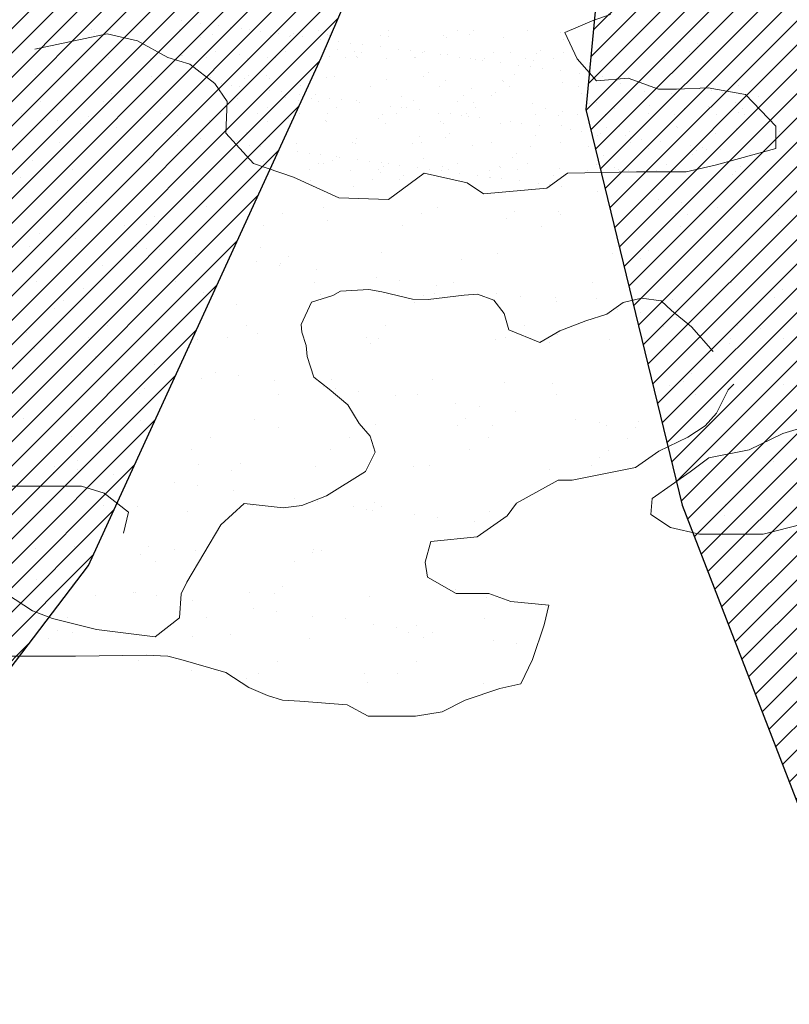
# Model space of a CAD drawing. Units: inches. Extents: x 1986 to 21484, y -1816 to 2016.
# Tile 13 of 85: x 2165 to 2172, y 1865 to 1874. Entities that reach past the tile are written whole.
import ezdxf

# ---------------------------------------------------------------- set-up
doc = ezdxf.new("R2010")
doc.units = ezdxf.units.IN
doc.layers.add('L-PLNT', color=84, linetype='Continuous', lineweight=13)
doc.layers.add('vfolhas', color=114, linetype='Continuous', lineweight=5)
for name, color, linetype in [('vfolha', 72, 'Continuous'), ('vfolha2', 110, 'Continuous'), ('vfolhas2', 102, 'Continuous')]:
    doc.layers.add(name, color=color, linetype=linetype)
pattern_1 = [(45, (-2446.5133113, 50.986076), (-0.004419417382, 0.004419417382), [])]

# ---------------------------------------------------------------- blocks, each defined once
blk = doc.blocks.new('arbusto_PB_verde_grande')
at = {"layer": 'vfolha2'}
h = blk.add_hatch(dxfattribs=at)
h.set_pattern_fill('ANSI31', color=256, scale=0.05, style=0)
h.set_pattern_definition(pattern_1)
h.paths.add_polyline_path([(0.02944, 0.35651), (0.00028, 0.09048), (0.02625, -0.03934), (0.047, 0.06233), (0.06189, 0.09731), (0.09372, 0.26573), (0.09955, 0.43473), (0.08789, 0.61313), (0.0645, 0.72266), (0.04988, 0.6851), (0.0236, 0.51294)])
h.paths.add_polyline_path([(0.30106, 0.43789), (0.14225, 0.24871), (0.26685, 0.30022)])
h.paths.add_polyline_path([(0.37995, 0.22817), (0.23697, 0.15193), (0.18428, 0.09364), (0.11122, 0.04358), (0.02625, -0.03934), (0.28061, 0.04667), (0.36829, 0.07798), (0.46756, 0.11239), (0.61068, 0.19376), (0.71585, 0.27823), (0.55813, 0.25948)])
h.paths.add_polyline_path([(0.56101, -0.29441), (0.72752, -0.32573), (0.59024, -0.2412), (0.42962, -0.15982), (0.02625, -0.03934), (0.14922, -0.14107), (0.18838, -0.16604), (0.41501, -0.24435)])
h.paths.add_polyline_path([(-0.27429, -0.44776), (-0.30352, -0.72628), (-0.23923, -0.64175), (-0.15457, -0.45716), (0.02625, -0.03934), (-0.16328, -0.25376)])
h.paths.add_polyline_path([(-0.51963, -0.24744), (-0.67736, -0.32573), (-0.59558, -0.35072), (-0.40574, -0.32882), (-0.21007, -0.20995), (0.02625, -0.03934), (-0.14874, -0.06595), (-0.31518, -0.09101), (-0.41452, -0.15048)])
h.paths.add_polyline_path([(-0.52546, 0.25007), (-0.70947, 0.24698), (-0.51963, 0.1093), (-0.32979, 0.02167), (-0.07567, -0.0128), (-0.04234, -0.02148), (-0.35024, 0.1312)])
at = {"layer": 'vfolhas'}
h = blk.add_hatch(dxfattribs=at)
h.set_pattern_fill('ANSI31', color=256, scale=0.05, style=0)
h.set_pattern_definition(pattern_1)
h.paths.add_polyline_path([(-0.07279, 0.50669), (-0.18085, 0.65063), (-0.2334, 0.67253), (-0.20712, 0.53176), (-0.10785, 0.25007), (0.02625, -0.03934), (0.00028, 0.09048), (0.00816, 0.16241), (-0.04939, 0.29079)])
h.paths.add_polyline_path([(0.09902, 0.41929), (0.09372, 0.26573), (0.07906, 0.18814), (0.15506, 0.36901), (0.26606, 0.5505), (0.28356, 0.63504), (0.2485, 0.68819), (0.25145, 0.63504), (0.20178, 0.54426)])
h.paths.add_polyline_path([(0.12295, 0.24073), (0.047, 0.06233), (0.02625, -0.03934), (0.11122, 0.04358), (0.18428, 0.09364), (0.27478, 0.19376), (0.3215, 0.25323), (0.44129, 0.38467), (0.47634, 0.57866), (0.41789, 0.45347), (0.28939, 0.30954)])
h.paths.add_polyline_path([(0.58145, -0.03779), (0.70707, 0.01536), (0.78591, 0.04667), (0.74796, 0.06549), (0.62818, 0.08423), (0.52595, 0.09048), (0.39745, 0.04358), (0.02625, -0.03934), (0.25728, -0.03154), (0.43834, -0.0347)])
h.paths.add_polyline_path([(0.52022, -0.03647), (0.43834, -0.0347), (0.25728, -0.03154), (0.02625, -0.03934), (0.17964, -0.08515), (0.53768, -0.13167), (0.69541, -0.15357), (0.78591, -0.07852), (0.70413, -0.10042)])
h.paths.add_polyline_path([(0.27189, -0.21929), (0.14922, -0.14107), (0.02625, -0.03934), (0.15794, -0.31007), (0.29522, -0.42585), (0.41789, -0.49157), (0.56396, -0.56669), (0.5114, -0.48532), (0.39456, -0.34139)])
h.paths.add_polyline_path([(-0.05818, -0.47591), (-0.02312, -0.61984), (0.047, -0.80134), (0.08494, -0.59794), (0.07911, -0.4071), (0.03527, -0.25376), (0.02625, -0.03934), (-0.03773, -0.26001)])
h.paths.add_polyline_path([(-0.24218, 0.14054), (-0.11073, 0.06858), (0.02625, -0.03934), (-0.04235, 0.10871), (-0.21007, 0.23757), (-0.36485, 0.33145), (-0.47874, 0.40341), (-0.54303, 0.46288), (-0.49041, 0.33145), (-0.39408, 0.22192)])
at = {"layer": 'vfolha'}
for p, q in [((-0.03773, -0.26001), (-0.05818, -0.47591)), ((-0.02312, -0.61984), (0.047, -0.80134))]:
    blk.add_line(p, q, dxfattribs=at)
at = {"layer": 'vfolha2'}
for p, q in [((-0.15457, -0.45716), (0.02625, -0.03934)), ((-0.30352, -0.72628), (-0.23923, -0.64175))]:
    blk.add_line(p, q, dxfattribs=at)
at = {"layer": 'vfolhas2'}
for p, q in [((-0.23923, -0.64175), (-0.15457, -0.45716)), ((-0.05818, -0.47591), (-0.02312, -0.61984))]:
    blk.add_line(p, q, dxfattribs=at)
blk = doc.blocks.new('PLANT-SHRUB')
for p, q in [((2166.5746, 1873.8887), (2166.5746, 1873.8887)), ((2170.0035, 1873.7837), (2170.2627, 1873.8946)), ((2170.2627, 1873.8946), (2170.4108, 1873.944)), ((2165.7672, 1873.807), (2165.7672, 1873.807)), ((2165.9347, 1873.8098), (2165.9347, 1873.8098)), ((2166.557, 1873.8087), (2166.557, 1873.8087)), ((2166.737, 1873.8673), (2166.737, 1873.8673)), ((2166.9045, 1873.8453), (2166.9045, 1873.8453)), ((2167.0085, 1873.8316), (2167.0085, 1873.8316)), ((2167.1125, 1873.8179), (2167.1125, 1873.8179)), ((2167.1125, 1873.8179), (2167.1125, 1873.8179)), ((2167.1794, 1873.8075), (2167.1794, 1873.8075)), ((2167.2749, 1873.7965), (2167.2749, 1873.7965)), ((2167.8017, 1873.8064), (2167.8017, 1873.8064)), ((2168.424, 1873.8053), (2168.424, 1873.8053)), ((2169.0463, 1873.8041), (2169.0463, 1873.8041)), ((2169.1885, 1873.8023), (2169.1885, 1873.8023)), ((2169.6686, 1873.803), (2169.6686, 1873.803)), ((2165.2583, 1873.6357), (2165.9062, 1873.7713)), ((2165.7957, 1873.7851), (2165.7957, 1873.7851)), ((2165.9062, 1873.7713), (2166.1777, 1873.7097)), ((2166.1777, 1873.7097), (2166.4493, 1873.5617)), ((2166.1777, 1873.7097), (2166.1777, 1873.7097)), ((2166.3069, 1873.7875), (2166.3069, 1873.7875)), ((2166.741, 1873.7371), (2166.741, 1873.7371)), ((2166.8467, 1873.7681), (2166.8467, 1873.7681)), ((2166.8467, 1873.7681), (2166.8467, 1873.7681)), ((2167.3697, 1873.7614), (2167.3697, 1873.7614)), ((2167.4374, 1873.7751), (2167.4374, 1873.7751)), ((2167.5406, 1873.744), (2167.5406, 1873.744)), ((2167.5464, 1873.7608), (2167.5464, 1873.7608)), ((2167.5774, 1873.7777), (2167.5774, 1873.7777)), ((2167.6504, 1873.7471), (2167.6504, 1873.7471)), ((2167.8129, 1873.7257), (2167.8129, 1873.7257)), ((2167.8809, 1873.7638), (2167.8809, 1873.7638)), ((2167.8928, 1873.7547), (2167.8928, 1873.7547)), ((2168.352, 1873.7617), (2168.352, 1873.7617)), ((2168.4207, 1873.7444), (2168.4207, 1873.7444)), ((2168.9152, 1873.7596), (2168.9152, 1873.7596)), ((2168.9438, 1873.7377), (2168.9438, 1873.7377)), ((2169.1516, 1873.7685), (2169.1516, 1873.7685)), ((2169.455, 1873.7402), (2169.455, 1873.7402)), ((2169.9631, 1873.7862), (2169.9631, 1873.7862)), ((2169.9947, 1873.7207), (2169.9947, 1873.7207)), ((2169.9947, 1873.7207), (2169.9947, 1873.7207)), ((2170.1146, 1873.5494), (2170.0035, 1873.7837)), ((2167.9692, 1873.6361), (2167.9692, 1873.6361)), ((2167.9803, 1873.7037), (2167.9803, 1873.7037)), ((2168.0843, 1873.69), (2168.0843, 1873.69)), ((2168.1883, 1873.6763), (2168.1883, 1873.6763)), ((2168.1883, 1873.6763), (2168.1883, 1873.6763)), ((2168.3508, 1873.6549), (2168.3508, 1873.6549)), ((2168.5132, 1873.6335), (2168.5132, 1873.6335)), ((2169.7892, 1873.6269), (2169.7892, 1873.6269)), ((2171.0409, 1873.7074), (2171.0409, 1873.7074)), ((2171.1913, 1873.6852), (2171.1913, 1873.6852)), ((2165.9152, 1873.5563), (2165.9152, 1873.5563)), ((2166.2963, 1873.5549), (2166.2963, 1873.5549)), ((2166.4493, 1873.5617), (2166.6467, 1873.5)), ((2166.5303, 1873.5441), (2166.5303, 1873.5441)), ((2166.5671, 1873.5778), (2166.5671, 1873.5778)), ((2166.5764, 1873.5807), (2166.5764, 1873.5807)), ((2166.7917, 1873.5606), (2166.7917, 1873.5606)), ((2166.876, 1873.6143), (2166.876, 1873.6143)), ((2167.0876, 1873.5831), (2167.0876, 1873.5831)), ((2167.1598, 1873.5541), (2167.1598, 1873.5541)), ((2167.3417, 1873.5617), (2167.3417, 1873.5617)), ((2167.414, 1873.5594), (2167.414, 1873.5594)), ((2167.4983, 1873.6131), (2167.4983, 1873.6131)), ((2167.6274, 1873.5637), (2167.6274, 1873.5637)), ((2167.8955, 1873.5686), (2167.8955, 1873.5686)), ((2168.0363, 1873.5583), (2168.0363, 1873.5583)), ((2168.1206, 1873.612), (2168.1206, 1873.612)), ((2168.1413, 1873.5686), (2168.1413, 1873.5686)), ((2168.1505, 1873.557), (2168.1505, 1873.557)), ((2168.1782, 1873.6023), (2168.1782, 1873.6023)), ((2168.4044, 1873.5518), (2168.4044, 1873.5518)), ((2168.6222, 1873.6192), (2168.6222, 1873.6192)), ((2168.6587, 1873.5572), (2168.6587, 1873.5572)), ((2168.6617, 1873.5595), (2168.6617, 1873.5595)), ((2168.7262, 1873.6055), (2168.7262, 1873.6055)), ((2168.7429, 1873.6109), (2168.7429, 1873.6109)), ((2168.8887, 1873.5841), (2168.8887, 1873.5841)), ((2168.9527, 1873.5863), (2168.9527, 1873.5863)), ((2169.0561, 1873.562), (2169.0561, 1873.562)), ((2169.1601, 1873.5483), (2169.1601, 1873.5483)), ((2169.2014, 1873.54), (2169.2014, 1873.54)), ((2169.2641, 1873.5346), (2169.2641, 1873.5346)), ((2169.2641, 1873.5346), (2169.2641, 1873.5346)), ((2169.281, 1873.556), (2169.281, 1873.556)), ((2169.3653, 1873.6097), (2169.3653, 1873.6097)), ((2169.5184, 1873.6039), (2169.5184, 1873.6039)), ((2169.6491, 1873.5495), (2169.6491, 1873.5495)), ((2169.7245, 1873.5334), (2169.7245, 1873.5334)), ((2169.7524, 1873.5931), (2169.7524, 1873.5931)), ((2169.9033, 1873.5549), (2169.9033, 1873.5549)), ((2169.9876, 1873.6086), (2169.9876, 1873.6086)), ((2170.1146, 1873.5494), (2170.1146, 1873.5494)), ((2170.2874, 1873.352), (2170.1146, 1873.5494)), ((2170.8937, 1873.5473), (2170.8937, 1873.5473)), ((2171.1176, 1873.6177), (2171.1176, 1873.6177)), ((2166.6467, 1873.5), (2166.8689, 1873.3274)), ((2169.4266, 1873.5133), (2169.4266, 1873.5133)), ((2169.5891, 1873.4919), (2169.5891, 1873.4919)), ((2169.698, 1873.4775), (2169.698, 1873.4775)), ((2169.802, 1873.4638), (2169.802, 1873.4638)), ((2165.2601, 1873.4067), (2165.2601, 1873.4067)), ((2166.3062, 1873.3933), (2166.3062, 1873.3933)), ((2166.8341, 1873.383), (2166.8341, 1873.383)), ((2167.131, 1873.3687), (2167.131, 1873.3687)), ((2167.1678, 1873.4024), (2167.1678, 1873.4024)), ((2167.3286, 1873.3982), (2167.3286, 1873.3982)), ((2167.3572, 1873.3763), (2167.3572, 1873.3763)), ((2167.8684, 1873.3788), (2167.8684, 1873.3788)), ((2167.9424, 1873.3863), (2167.9424, 1873.3863)), ((2168.4081, 1873.3593), (2168.4081, 1873.3593)), ((2168.4081, 1873.3593), (2168.4081, 1873.3593)), ((2168.742, 1873.3932), (2168.742, 1873.3932)), ((2168.7789, 1873.427), (2168.7789, 1873.427)), ((2169.5535, 1873.4109), (2169.5535, 1873.4109)), ((2169.9645, 1873.4424), (2169.9645, 1873.4424)), ((2170.1319, 1873.4204), (2170.1319, 1873.4204)), ((2170.2359, 1873.4067), (2170.2359, 1873.4067)), ((2170.5712, 1873.3767), (2170.2874, 1873.352)), ((2170.34, 1873.393), (2170.34, 1873.393)), ((2170.8427, 1873.2781), (2170.5712, 1873.3767)), ((2166.8689, 1873.3274), (2166.9799, 1873.1671)), ((2166.9282, 1873.3248), (2166.9282, 1873.3248)), ((2167.018, 1873.3071), (2167.018, 1873.3071)), ((2167.0907, 1873.3034), (2167.0907, 1873.3034)), ((2167.3621, 1873.2676), (2167.3621, 1873.2676)), ((2167.6403, 1873.306), (2167.6403, 1873.306)), ((2168.2626, 1873.3049), (2168.2626, 1873.3049)), ((2168.8849, 1873.3037), (2168.8849, 1873.3037)), ((2168.9312, 1873.3527), (2168.9312, 1873.3527)), ((2169.1706, 1873.2853), (2169.1706, 1873.2853)), ((2169.4424, 1873.3551), (2169.4424, 1873.3551)), ((2169.4543, 1873.346), (2169.4543, 1873.346)), ((2169.5072, 1873.3026), (2169.5072, 1873.3026)), ((2169.9821, 1873.3357), (2169.9821, 1873.3357)), ((2170.1295, 1873.3015), (2170.1295, 1873.3015)), ((2170.4767, 1873.3509), (2170.4767, 1873.3509)), ((2170.5052, 1873.329), (2170.5052, 1873.329)), ((2170.6649, 1873.3502), (2170.6649, 1873.3502)), ((2170.7519, 1873.3003), (2170.7519, 1873.3003)), ((2171.0032, 1873.2781), (2170.8427, 1873.2781)), ((2170.9907, 1873.2761), (2170.9907, 1873.2761)), ((2171.287, 1873.2904), (2171.0032, 1873.2781)), ((2171.2077, 1873.2788), (2171.2077, 1873.2788)), ((2171.6202, 1873.2287), (2171.287, 1873.2904)), ((2171.5561, 1873.312), (2171.5561, 1873.312)), ((2165.9485, 1873.2362), (2165.9485, 1873.2362)), ((2167.0751, 1873.1981), (2167.0751, 1873.1981)), ((2167.4661, 1873.254), (2167.4661, 1873.254)), ((2167.4977, 1873.2041), (2167.4977, 1873.2041)), ((2167.6286, 1873.2326), (2167.6286, 1873.2326)), ((2167.7317, 1873.1933), (2167.7317, 1873.1933)), ((2167.7686, 1873.227), (2167.7686, 1873.227)), ((2167.9, 1873.1968), (2167.9, 1873.1968)), ((2168.0041, 1873.1831), (2168.0041, 1873.1831)), ((2168.5431, 1873.2109), (2168.5431, 1873.2109)), ((2169.097, 1873.2178), (2169.097, 1873.2178)), ((2169.3428, 1873.2178), (2169.3428, 1873.2178)), ((2169.3796, 1873.2516), (2169.3796, 1873.2516)), ((2170.1542, 1873.2355), (2170.1542, 1873.2355)), ((2170.7198, 1873.2532), (2170.7198, 1873.2532)), ((2170.9538, 1873.2424), (2170.9538, 1873.2424)), ((2171.3118, 1873.2651), (2171.3118, 1873.2651)), ((2171.4158, 1873.2514), (2171.4158, 1873.2514)), ((2171.4158, 1873.2514), (2171.4158, 1873.2514)), ((2171.5782, 1873.23), (2171.5782, 1873.23)), ((2171.8918, 1872.9451), (2171.6202, 1873.2287)), ((2171.7407, 1873.2086), (2171.7407, 1873.2086)), ((2165.3084, 1873.1698), (2165.3084, 1873.1698)), ((2165.8749, 1873.1687), (2165.8749, 1873.1687)), ((2166.5531, 1873.1675), (2166.5531, 1873.1675)), ((2166.9799, 1873.1671), (2166.9676, 1872.8834)), ((2167.3369, 1873.1127), (2167.3369, 1873.1127)), ((2167.6148, 1873.1787), (2167.6148, 1873.1787)), ((2167.7977, 1873.1653), (2167.7977, 1873.1653)), ((2167.9592, 1873.1116), (2167.9592, 1873.1116)), ((2168.1379, 1873.172), (2168.1379, 1873.172)), ((2168.1665, 1873.1617), (2168.1665, 1873.1617)), ((2168.438, 1873.126), (2168.438, 1873.126)), ((2168.542, 1873.1123), (2168.542, 1873.1123)), ((2168.5815, 1873.1105), (2168.5815, 1873.1105)), ((2168.6491, 1873.1744), (2168.6491, 1873.1744)), ((2168.7044, 1873.0909), (2168.7044, 1873.0909)), ((2169.0423, 1873.163), (2169.0423, 1873.163)), ((2169.1888, 1873.155), (2169.1888, 1873.155)), ((2169.2039, 1873.1093), (2169.2039, 1873.1093)), ((2169.7119, 1873.1483), (2169.7119, 1873.1483)), ((2169.8262, 1873.1082), (2169.8262, 1873.1082)), ((2170.2231, 1873.1508), (2170.2231, 1873.1508)), ((2170.287, 1873.1607), (2170.287, 1873.1607)), ((2170.4485, 1873.1071), (2170.4485, 1873.1071)), ((2170.7628, 1873.1313), (2170.7628, 1873.1313)), ((2171.0708, 1873.1059), (2171.0708, 1873.1059)), ((2171.2859, 1873.1247), (2171.2859, 1873.1247)), ((2171.5316, 1873.1585), (2171.5316, 1873.1585)), ((2171.5914, 1873.1007), (2171.5914, 1873.1007)), ((2165.1399, 1873.0624), (2165.1399, 1873.0624)), ((2165.742, 1873.0369), (2165.742, 1873.0369)), ((2166.3845, 1873.0602), (2166.3845, 1873.0602)), ((2167.2526, 1873.059), (2167.2526, 1873.059)), ((2167.5328, 1873.011), (2167.5328, 1873.011)), ((2167.6292, 1873.0579), (2167.6292, 1873.0579)), ((2167.875, 1873.0579), (2167.875, 1873.0579)), ((2168.3325, 1873.0179), (2168.3325, 1873.0179)), ((2168.3693, 1873.0516), (2168.3693, 1873.0516)), ((2168.4973, 1873.0568), (2168.4973, 1873.0568)), ((2168.8738, 1873.0556), (2168.8738, 1873.0556)), ((2168.9759, 1873.0552), (2168.9759, 1873.0552)), ((2169.0799, 1873.0415), (2169.0799, 1873.0415)), ((2169.1196, 1873.0556), (2169.1196, 1873.0556)), ((2169.1439, 1873.0356), (2169.1439, 1873.0356)), ((2169.2423, 1873.0201), (2169.2423, 1873.0201)), ((2169.7419, 1873.0545), (2169.7419, 1873.0545)), ((2169.9435, 1873.0424), (2169.9435, 1873.0424)), ((2169.9803, 1873.0762), (2169.9803, 1873.0762)), ((2170.1184, 1873.0534), (2170.1184, 1873.0534)), ((2170.3642, 1873.0534), (2170.3642, 1873.0534)), ((2170.7549, 1873.0601), (2170.7549, 1873.0601)), ((2170.9865, 1873.0522), (2170.9865, 1873.0522)), ((2171.3631, 1873.0511), (2171.3631, 1873.0511)), ((2171.5546, 1873.067), (2171.5546, 1873.067)), ((2171.6089, 1873.0511), (2171.6089, 1873.0511)), ((2165.4601, 1873.0006), (2165.4601, 1873.0006)), ((2165.6682, 1872.9733), (2165.6682, 1872.9733)), ((2165.9931, 1872.9305), (2165.9931, 1872.9305)), ((2166.8215, 1872.998), (2166.8215, 1872.998)), ((2167.3446, 1872.9913), (2167.3446, 1872.9913)), ((2167.8558, 1872.9937), (2167.8558, 1872.9937)), ((2167.8677, 1872.9846), (2167.8677, 1872.9846)), ((2168.3955, 1872.9743), (2168.3955, 1872.9743)), ((2168.8901, 1872.9895), (2168.8901, 1872.9895)), ((2168.9186, 1872.9676), (2168.9186, 1872.9676)), ((2169.4298, 1872.9701), (2169.4298, 1872.9701)), ((2169.5138, 1872.9844), (2169.5138, 1872.9844)), ((2169.6178, 1872.9707), (2169.6178, 1872.9707)), ((2169.7803, 1872.9493), (2169.7803, 1872.9493)), ((2169.9695, 1872.9506), (2169.9695, 1872.9506)), ((2169.9695, 1872.9506), (2169.9695, 1872.9506)), ((2170.3721, 1872.9345), (2170.3721, 1872.9345)), ((2170.4926, 1872.944), (2170.4926, 1872.944)), ((2171.0038, 1872.9464), (2171.0038, 1872.9464)), ((2171.0157, 1872.9373), (2171.0157, 1872.9373)), ((2171.5435, 1872.927), (2171.5435, 1872.927)), ((2171.8918, 1872.7478), (2171.8918, 1872.9451)), ((2166.536, 1872.859), (2166.536, 1872.859)), ((2166.744, 1872.8316), (2166.744, 1872.8316)), ((2166.9676, 1872.8834), (2167.2144, 1872.6121)), ((2167.15, 1872.8855), (2167.15, 1872.8855)), ((2167.359, 1872.8517), (2167.359, 1872.8517)), ((2168.1336, 1872.8356), (2168.1336, 1872.8356)), ((2168.6992, 1872.8533), (2168.6992, 1872.8533)), ((2168.9332, 1872.8425), (2168.9332, 1872.8425)), ((2168.97, 1872.8762), (2168.97, 1872.8762)), ((2169.7446, 1872.8602), (2169.7446, 1872.8602)), ((2170.0517, 1872.9136), (2170.0517, 1872.9136)), ((2170.1557, 1872.8999), (2170.1557, 1872.8999)), ((2170.2984, 1872.867), (2170.2984, 1872.867)), ((2170.3182, 1872.8785), (2170.3182, 1872.8785)), ((2170.5442, 1872.867), (2170.5442, 1872.867)), ((2170.5811, 1872.9008), (2170.5811, 1872.9008)), ((2170.5896, 1872.8427), (2170.5896, 1872.8427)), ((2170.6936, 1872.829), (2170.6936, 1872.829)), ((2171.3557, 1872.8847), (2171.3557, 1872.8847)), ((2171.9213, 1872.9024), (2171.9213, 1872.9024)), ((2165.4771, 1872.8042), (2165.4771, 1872.8042)), ((2167.0625, 1872.8131), (2167.0625, 1872.8131)), ((2167.0689, 1872.7888), (2167.0689, 1872.7888)), ((2167.0763, 1872.818), (2167.0763, 1872.818)), ((2167.1779, 1872.7745), (2167.1779, 1872.7745)), ((2167.2819, 1872.7608), (2167.2819, 1872.7608)), ((2167.3221, 1872.818), (2167.3221, 1872.818)), ((2167.4444, 1872.7394), (2167.4444, 1872.7394)), ((2167.4789, 1872.8056), (2167.4789, 1872.8056)), ((2167.6022, 1872.7936), (2167.6022, 1872.7936)), ((2168.1012, 1872.8044), (2168.1012, 1872.8044)), ((2168.1253, 1872.7869), (2168.1253, 1872.7869)), ((2168.6365, 1872.7894), (2168.6365, 1872.7894)), ((2168.7235, 1872.8033), (2168.7235, 1872.8033)), ((2169.1762, 1872.7699), (2169.1762, 1872.7699)), ((2169.3458, 1872.8022), (2169.3458, 1872.8022)), ((2169.6993, 1872.7633), (2169.6993, 1872.7633)), ((2169.9682, 1872.8011), (2169.9682, 1872.8011)), ((2170.2105, 1872.7657), (2170.2105, 1872.7657)), ((2170.5905, 1872.7999), (2170.5905, 1872.7999)), ((2170.7502, 1872.7463), (2170.7502, 1872.7463)), ((2170.8561, 1872.8077), (2170.8561, 1872.8077)), ((2171.1275, 1872.7719), (2171.1275, 1872.7719)), ((2171.2128, 1872.7988), (2171.2128, 1872.7988)), ((2171.2315, 1872.7582), (2171.2315, 1872.7582)), ((2171.2733, 1872.7396), (2171.2733, 1872.7396)), ((2171.3611, 1872.5998), (2171.8918, 1872.7478)), ((2167.6118, 1872.7174), (2167.6118, 1872.7174)), ((2167.7158, 1872.7037), (2167.7158, 1872.7037)), ((2167.8198, 1872.69), (2167.8198, 1872.69)), ((2167.8198, 1872.69), (2167.8198, 1872.69)), ((2167.9597, 1872.6763), (2167.9597, 1872.6763)), ((2167.9823, 1872.6686), (2167.9823, 1872.6686)), ((2168.7343, 1872.6602), (2168.7343, 1872.6602)), ((2169.5339, 1872.6671), (2169.5339, 1872.6671)), ((2169.5708, 1872.7009), (2169.5708, 1872.7009)), ((2170.3453, 1872.6848), (2170.3453, 1872.6848)), ((2171.145, 1872.6916), (2171.145, 1872.6916)), ((2171.1818, 1872.7254), (2171.1818, 1872.7254)), ((2171.394, 1872.7368), (2171.394, 1872.7368)), ((2171.6654, 1872.7011), (2171.6654, 1872.7011)), ((2165.2349, 1872.6366), (2165.2349, 1872.6366)), ((2166.2811, 1872.6232), (2166.2811, 1872.6232)), ((2167.2144, 1872.6121), (2167.5723, 1872.4888)), ((2167.2144, 1872.6121), (2167.2144, 1872.6121)), ((2167.3034, 1872.6281), (2167.3034, 1872.6281)), ((2167.332, 1872.6062), (2167.332, 1872.6062)), ((2167.7978, 1872.6112), (2167.7978, 1872.6112)), ((2167.8432, 1872.6087), (2167.8432, 1872.6087)), ((2167.9229, 1872.6426), (2167.9229, 1872.6426)), ((2168.1447, 1872.6472), (2168.1447, 1872.6472)), ((2168.2537, 1872.6329), (2168.2537, 1872.6329)), ((2168.3577, 1872.6192), (2168.3577, 1872.6192)), ((2168.3829, 1872.5893), (2168.3829, 1872.5893)), ((2168.3829, 1872.5893), (2168.3829, 1872.5893)), ((2168.4201, 1872.61), (2168.4201, 1872.61)), ((2168.5202, 1872.5978), (2168.5202, 1872.5978)), ((2168.6876, 1872.5757), (2168.6876, 1872.5757)), ((2168.906, 1872.5826), (2168.906, 1872.5826)), ((2169.0425, 1872.6089), (2169.0425, 1872.6089)), ((2169.4172, 1872.585), (2169.4172, 1872.585)), ((2169.4291, 1872.5759), (2169.4291, 1872.5759)), ((2169.6648, 1872.6078), (2169.6648, 1872.6078)), ((2169.9569, 1872.5656), (2169.9569, 1872.5656)), ((2170.2871, 1872.6067), (2170.2871, 1872.6067)), ((2170.4515, 1872.5808), (2170.4515, 1872.5808)), ((2170.9094, 1872.6055), (2170.9094, 1872.6055)), ((2171.0896, 1872.5382), (2171.3611, 1872.5998)), ((2171.5736, 1872.5838), (2171.5736, 1872.5838)), ((2165.1294, 1872.4856), (2165.1294, 1872.4856)), ((2165.5924, 1872.5555), (2165.5924, 1872.5555)), ((2166.837, 1872.5533), (2166.837, 1872.5533)), ((2167.5723, 1872.4888), (2167.9796, 1872.3039)), ((2167.7136, 1872.5575), (2167.7136, 1872.5575)), ((2168.0817, 1872.551), (2168.0817, 1872.551)), ((2168.3359, 1872.5564), (2168.3359, 1872.5564)), ((2168.3515, 1872.5347), (2168.3515, 1872.5347)), ((2168.4239, 1872.2915), (2168.7447, 1872.5258)), ((2168.5604, 1872.5009), (2168.5604, 1872.5009)), ((2168.7447, 1872.5258), (2169.1273, 1872.4395)), ((2168.7916, 1872.562), (2168.7916, 1872.562)), ((2168.8956, 1872.5484), (2168.8956, 1872.5484)), ((2168.8956, 1872.5484), (2168.8956, 1872.5484)), ((2168.9582, 1872.5552), (2168.9582, 1872.5552)), ((2169.0581, 1872.527), (2169.0581, 1872.527)), ((2169.2206, 1872.5056), (2169.2206, 1872.5056)), ((2169.3263, 1872.5487), (2169.3263, 1872.5487)), ((2169.3295, 1872.4912), (2169.3295, 1872.4912)), ((2169.335, 1872.4848), (2169.335, 1872.4848)), ((2169.4335, 1872.4775), (2169.4335, 1872.4775)), ((2169.5805, 1872.5541), (2169.5805, 1872.5541)), ((2169.8431, 1872.3902), (2170.0282, 1872.5258)), ((2169.9006, 1872.5025), (2169.9006, 1872.5025)), ((2170.0282, 1872.5258), (2170.6453, 1872.5382)), ((2170.2028, 1872.553), (2170.2028, 1872.553)), ((2170.48, 1872.5589), (2170.48, 1872.5589)), ((2170.5709, 1872.5465), (2170.5709, 1872.5465)), ((2170.6453, 1872.5382), (2171.0896, 1872.5382)), ((2170.8251, 1872.5518), (2170.8251, 1872.5518)), ((2170.9912, 1872.5614), (2170.9912, 1872.5614)), ((2171.4999, 1872.5163), (2171.4999, 1872.5163)), ((2171.531, 1872.5419), (2171.531, 1872.5419)), ((2171.8156, 1872.5442), (2171.8156, 1872.5442)), ((2166.6785, 1872.4534), (2166.6785, 1872.4534)), ((2167.724, 1872.4603), (2167.724, 1872.4603)), ((2168.1127, 1872.4019), (2168.1127, 1872.4019)), ((2168.2778, 1872.4672), (2168.2778, 1872.4672)), ((2168.5236, 1872.4672), (2168.5236, 1872.4672)), ((2169.1273, 1872.4395), (2169.2754, 1872.3408)), ((2169.2754, 1872.3408), (2169.8431, 1872.3902)), ((2169.596, 1872.4561), (2169.596, 1872.4561)), ((2169.7634, 1872.4341), (2169.7634, 1872.4341)), ((2169.8674, 1872.4204), (2169.8674, 1872.4204)), ((2169.9715, 1872.4067), (2169.9715, 1872.4067)), ((2167.9796, 1872.3039), (2168.4239, 1872.2915)), ((2169.6867, 1872.3782), (2169.6867, 1872.3782)), ((2170.2964, 1872.3639), (2170.2964, 1872.3639)), ((2165.7168, 1872.2668), (2165.7168, 1872.2668)), ((2166.7963, 1872.2279), (2166.7963, 1872.2279)), ((2167.8425, 1872.2145), (2167.8425, 1872.2145)), ((2168.8649, 1872.2194), (2168.8649, 1872.2194)), ((2170.8393, 1872.2925), (2170.8393, 1872.2925)), ((2171.0473, 1872.2651), (2171.0473, 1872.2651)), ((2171.3722, 1872.2223), (2171.3722, 1872.2223)), ((2166.2303, 1872.1667), (2166.2303, 1872.1667)), ((2166.3308, 1872.1348), (2166.3308, 1872.1348)), ((2167.4749, 1872.1645), (2167.4749, 1872.1645)), ((2168.7195, 1872.1622), (2168.7195, 1872.1622)), ((2169.5529, 1872.1839), (2169.5529, 1872.1839)), ((2169.9443, 1872.1805), (2169.9443, 1872.1805)), ((2169.9642, 1872.1599), (2169.9642, 1872.1599)), ((2170.9905, 1872.1672), (2170.9905, 1872.1672)), ((2171.1021, 1872.1517), (2171.1021, 1872.1517)), ((2171.2088, 1872.1577), (2171.2088, 1872.1577)), ((2171.9151, 1872.1508), (2171.9151, 1872.1508)), ((2166.0617, 1872.0593), (2166.0617, 1872.0593)), ((2166.2572, 1872.0673), (2166.2572, 1872.0673)), ((2167.3064, 1872.0571), (2167.3064, 1872.0571)), ((2167.88, 1872.1027), (2167.88, 1872.1027)), ((2168.551, 1872.0548), (2168.551, 1872.0548)), ((2169.4793, 1872.1164), (2169.4793, 1872.1164)), ((2169.7956, 1872.0526), (2169.7956, 1872.0526)), ((2171.0403, 1872.0503), (2171.0403, 1872.0503)), ((2165.2997, 1871.987), (2165.2997, 1871.987)), ((2165.2097, 1871.8665), (2165.2097, 1871.8665)), ((2165.6246, 1871.9442), (2165.6246, 1871.9442)), ((2166.1675, 1871.8727), (2166.1675, 1871.8727)), ((2167.2783, 1871.858), (2167.2783, 1871.858)), ((2166.2559, 1871.8531), (2166.2559, 1871.8531)), ((2166.3755, 1871.8453), (2166.3755, 1871.8453)), ((2166.7004, 1871.8025), (2166.7004, 1871.8025)), ((2167.5323, 1871.784), (2167.5323, 1871.784)), ((2168.3577, 1871.8192), (2168.3577, 1871.8192)), ((2169.4039, 1871.8058), (2169.4039, 1871.8058)), ((2170.4263, 1871.8107), (2170.4263, 1871.8107)), ((2170.7544, 1871.8331), (2170.7544, 1871.8331)), ((2171.5058, 1871.7718), (2171.5058, 1871.7718)), ((2165.8594, 1871.7028), (2165.8594, 1871.7028)), ((2167.2433, 1871.7311), (2167.2433, 1871.7311)), ((2167.4513, 1871.7037), (2167.4513, 1871.7037)), ((2167.4586, 1871.7165), (2167.4586, 1871.7165)), ((2169.0815, 1871.7519), (2169.0815, 1871.7519)), ((2170.6807, 1871.7656), (2170.6807, 1871.7656)), ((2167.7762, 1871.6609), (2167.7762, 1871.6609)), ((2165.2696, 1871.5547), (2165.2696, 1871.5547)), ((2166.5142, 1871.5524), (2166.5142, 1871.5524)), ((2167.7589, 1871.5502), (2167.7589, 1871.5502)), ((2168.3191, 1871.5894), (2168.3191, 1871.5894)), ((2168.5271, 1871.5621), (2168.5271, 1871.5621)), ((2168.8521, 1871.5193), (2168.8521, 1871.5193)), ((2169.0035, 1871.5479), (2169.0035, 1871.5479)), ((2170.2481, 1871.5457), (2170.2481, 1871.5457)), ((2171.4928, 1871.5434), (2171.4928, 1871.5434)), ((2165.6917, 1871.4967), (2165.6917, 1871.4967)), ((2166.7711, 1871.4578), (2166.7711, 1871.4578)), ((2167.7351, 1871.3723), (2167.9246, 1871.4318)), ((2167.8173, 1871.4444), (2167.8173, 1871.4444)), ((2167.9246, 1871.4318), (2167.995, 1871.4697)), ((2167.995, 1871.4697), (2168.2495, 1871.4859)), ((2168.2495, 1871.4859), (2168.3632, 1871.4643)), ((2168.3632, 1871.4643), (2168.6394, 1871.3994)), ((2168.7338, 1871.4333), (2168.7338, 1871.4333)), ((2168.7801, 1871.394), (2169.1015, 1871.4329)), ((2168.8397, 1871.4493), (2168.8397, 1871.4493)), ((2169.1015, 1871.4329), (2169.2206, 1871.4437)), ((2169.2206, 1871.4437), (2169.3668, 1871.3896)), ((2169.3949, 1871.4478), (2169.3949, 1871.4478)), ((2169.603, 1871.4204), (2169.603, 1871.4204)), ((2171.9559, 1871.4823), (2171.9559, 1871.4823)), ((2165.5117, 1871.3842), (2165.5117, 1871.3842)), ((2167.0608, 1871.352), (2167.0608, 1871.352)), ((2167.643, 1871.1721), (2167.7351, 1871.3723)), ((2168.6394, 1871.3994), (2168.7801, 1871.394)), ((2168.6601, 1871.3658), (2168.6601, 1871.3658)), ((2169.3668, 1871.3896), (2169.4589, 1871.2705)), ((2169.9192, 1871.4104), (2169.9192, 1871.4104)), ((2169.9279, 1871.3776), (2169.9279, 1871.3776)), ((2170.2829, 1871.4011), (2170.2829, 1871.4011)), ((2170.3794, 1871.2651), (2170.5256, 1871.3679)), ((2170.5256, 1871.3679), (2170.6881, 1871.4058)), ((2170.6881, 1871.4058), (2170.8667, 1871.3842)), ((2170.8667, 1871.3842), (2170.9588, 1871.2976)), ((2170.9653, 1871.3971), (2170.9653, 1871.3971)), ((2171.8822, 1871.4148), (2171.8822, 1871.4148)), ((2171.9877, 1871.402), (2171.9877, 1871.402)), ((2165.438, 1871.3167), (2165.438, 1871.3167)), ((2169.4589, 1871.2705), (2169.5022, 1871.1244)), ((2170.1899, 1871.2056), (2170.3794, 1871.2651)), ((2170.4708, 1871.3062), (2170.4708, 1871.3062)), ((2170.6788, 1871.2788), (2170.6788, 1871.2788)), ((2170.9588, 1871.2976), (2171.1375, 1871.1515)), ((2165.9075, 1871.1659), (2165.9075, 1871.1659)), ((2167.1521, 1871.1636), (2167.1521, 1871.1636)), ((2167.6484, 1871.1018), (2167.643, 1871.1721)), ((2168.3968, 1871.1614), (2168.3968, 1871.1614)), ((2169.6414, 1871.1591), (2169.6414, 1871.1591)), ((2169.9571, 1871.1136), (2170.1899, 1871.2056)), ((2170.886, 1871.1569), (2170.886, 1871.1569)), ((2171.0037, 1871.236), (2171.0037, 1871.236)), ((2171.5466, 1871.1645), (2171.5466, 1871.1645)), ((2165.1845, 1871.0964), (2165.1845, 1871.0964)), ((2166.2307, 1871.083), (2166.2307, 1871.083)), ((2167.2531, 1871.0879), (2167.2531, 1871.0879)), ((2167.6863, 1870.9827), (2167.6484, 1871.1018)), ((2169.5022, 1871.1244), (2169.7784, 1871.0108)), ((2169.7784, 1871.0108), (2169.9571, 1871.1136)), ((2169.9352, 1871.0825), (2169.9352, 1871.0825)), ((2171.1375, 1871.1515), (2171.3324, 1870.9297)), ((2171.7546, 1871.1372), (2171.7546, 1871.1372)), ((2165.739, 1871.0585), (2165.739, 1871.0585)), ((2166.7131, 1871.0334), (2166.7131, 1871.0334)), ((2166.9836, 1871.0563), (2166.9836, 1871.0563)), ((2167.6972, 1870.8854), (2167.6863, 1870.9827)), ((2168.2282, 1871.054), (2168.2282, 1871.054)), ((2168.2623, 1871.0012), (2168.2623, 1871.0012)), ((2168.3326, 1871.0491), (2168.3326, 1871.0491)), ((2169.3787, 1871.0357), (2169.3787, 1871.0357)), ((2169.4729, 1871.0517), (2169.4729, 1871.0517)), ((2169.8616, 1871.015), (2169.8616, 1871.015)), ((2170.4011, 1871.0406), (2170.4011, 1871.0406)), ((2170.7175, 1871.0495), (2170.7175, 1871.0495)), ((2171.4806, 1871.0017), (2171.4806, 1871.0017)), ((2171.4844, 1871.0503), (2171.4844, 1871.0503)), ((2171.9621, 1871.0472), (2171.9621, 1871.0472)), ((2165.2561, 1870.9579), (2165.2561, 1870.9579)), ((2166.6394, 1870.9659), (2166.6394, 1870.9659)), ((2165.799, 1870.8864), (2165.799, 1870.8864)), ((2166.007, 1870.859), (2166.007, 1870.859)), ((2166.3319, 1870.8163), (2166.3319, 1870.8163)), ((2167.7567, 1870.7014), (2167.6972, 1870.8854)), ((2165.6665, 1870.7266), (2165.6665, 1870.7266)), ((2166.8748, 1870.7448), (2166.8748, 1870.7448)), ((2167.0828, 1870.7174), (2167.0828, 1870.7174)), ((2171.1367, 1870.7317), (2171.1367, 1870.7317)), ((2166.746, 1870.6877), (2166.746, 1870.6877)), ((2167.4077, 1870.6746), (2167.4077, 1870.6746)), ((2167.8921, 1870.5932), (2167.7567, 1870.7014)), ((2167.7921, 1870.6743), (2167.7921, 1870.6743)), ((2167.9146, 1870.6826), (2167.9146, 1870.6826)), ((2168.8145, 1870.6792), (2168.8145, 1870.6792)), ((2169.4637, 1870.6505), (2169.4637, 1870.6505)), ((2169.894, 1870.6403), (2169.894, 1870.6403)), ((2170.9402, 1870.627), (2170.9402, 1870.627)), ((2171.063, 1870.6642), (2171.063, 1870.6642)), ((2171.5171, 1870.6384), (2171.4653, 1870.5867)), ((2171.9626, 1870.6319), (2171.9626, 1870.6319)), ((2166.1915, 1870.5516), (2166.1915, 1870.5516)), ((2166.2416, 1870.6014), (2166.2416, 1870.6014)), ((2167.4361, 1870.5494), (2167.4361, 1870.5494)), ((2167.8409, 1870.6151), (2167.8409, 1870.6151)), ((2168.06, 1870.4525), (2167.8921, 1870.5932)), ((2167.9506, 1870.6031), (2167.9506, 1870.6031)), ((2168.1586, 1870.5758), (2168.1586, 1870.5758)), ((2168.6807, 1870.5471), (2168.6807, 1870.5471)), ((2169.9254, 1870.5448), (2169.9254, 1870.5448)), ((2171.17, 1870.5426), (2171.17, 1870.5426)), ((2171.4653, 1870.5867), (2171.3617, 1870.3797)), ((2168.1629, 1870.2848), (2168.06, 1870.4525)), ((2168.4836, 1870.533), (2168.4836, 1870.533)), ((2169.0264, 1870.4615), (2169.0264, 1870.4615)), ((2169.2345, 1870.4341), (2169.2345, 1870.4341)), ((2169.5594, 1870.3913), (2169.5594, 1870.3913)), ((2171.3617, 1870.3797), (2171.2581, 1870.2658)), ((2165.1593, 1870.3263), (2165.1593, 1870.3263)), ((2165.8939, 1870.2828), (2165.8939, 1870.2828)), ((2166.2055, 1870.313), (2166.2055, 1870.313)), ((2167.2279, 1870.3179), (2167.2279, 1870.3179)), ((2168.2603, 1870.1712), (2168.1629, 1870.2848)), ((2168.3074, 1870.279), (2168.3074, 1870.279)), ((2169.116, 1870.3318), (2169.116, 1870.3318)), ((2170.1023, 1870.3199), (2170.1023, 1870.3199)), ((2170.3103, 1870.2925), (2170.3103, 1870.2925)), ((2170.6652, 1870.2997), (2170.6652, 1870.2997)), ((2165.8203, 1870.2153), (2165.8203, 1870.2153)), ((2167.4431, 1870.2506), (2167.4431, 1870.2506)), ((2169.0424, 1870.2643), (2169.0424, 1870.2643)), ((2169.3536, 1870.2656), (2169.3536, 1870.2656)), ((2170.376, 1870.2705), (2170.376, 1870.2705)), ((2170.6352, 1870.2497), (2170.6352, 1870.2497)), ((2171.2581, 1870.2658), (2171.1028, 1870.1623)), ((2171.6537, 1870.0501), (2171.9541, 1870.195)), ((2171.9541, 1870.195), (2172.1923, 1870.2675)), ((2165.5847, 1870.1651), (2165.5847, 1870.1651)), ((2166.8293, 1870.1628), (2166.8293, 1870.1628)), ((2168.074, 1870.1606), (2168.074, 1870.1606)), ((2168.3036, 1870.0305), (2168.2603, 1870.1712)), ((2169.3186, 1870.1583), (2169.3186, 1870.1583)), ((2170.5632, 1870.156), (2170.5632, 1870.156)), ((2171.1028, 1870.1623), (2170.8439, 1870.0382)), ((2165.4162, 1870.0577), (2165.4162, 1870.0577)), ((2166.6608, 1870.0554), (2166.6608, 1870.0554)), ((2167.9054, 1870.0532), (2167.9054, 1870.0532)), ((2168.217, 1869.8573), (2168.3036, 1870.0305)), ((2169.1501, 1870.0509), (2169.1501, 1870.0509)), ((2170.3947, 1870.0487), (2170.3947, 1870.0487)), ((2170.8439, 1870.0382), (2170.6367, 1869.8933)), ((2171.2912, 1869.9777), (2171.6537, 1870.0501)), ((2171.6393, 1870.0464), (2171.6393, 1870.0464)), ((2171.6537, 1870.0501), (2171.6537, 1870.0501)), ((2165.6413, 1869.9565), (2165.6413, 1869.9565)), ((2167.0954, 1869.932), (2167.0954, 1869.932)), ((2170.3175, 1869.9811), (2170.3175, 1869.9811)), ((2171.1255, 1869.8535), (2171.2912, 1869.9777)), ((2171.8667, 1869.9489), (2171.8667, 1869.9489)), ((2165.4225, 1869.8507), (2165.4225, 1869.8507)), ((2165.4305, 1869.9001), (2165.4305, 1869.9001)), ((2165.6385, 1869.8727), (2165.6385, 1869.8727)), ((2166.7208, 1869.9176), (2166.7208, 1869.9176)), ((2167.0217, 1869.8645), (2167.0217, 1869.8645)), ((2167.767, 1869.9042), (2167.767, 1869.9042)), ((2167.8695, 1869.6393), (2168.217, 1869.8573)), ((2168.6446, 1869.8998), (2168.6446, 1869.8998)), ((2168.7893, 1869.9091), (2168.7893, 1869.9091)), ((2169.8688, 1869.8702), (2169.8688, 1869.8702)), ((2170.6367, 1869.8933), (2170.0671, 1869.7794)), ((2170.2438, 1869.9136), (2170.2438, 1869.9136)), ((2170.7837, 1869.6155), (2171.1255, 1869.8535)), ((2171.1255, 1869.8535), (2171.1255, 1869.8535)), ((2171.9374, 1869.8618), (2171.9374, 1869.8618)), ((2165.9634, 1869.83), (2165.9634, 1869.83)), ((2166.5063, 1869.7585), (2166.5063, 1869.7585)), ((2169.9428, 1869.7794), (2169.5699, 1869.5724)), ((2170.0671, 1869.7794), (2169.9428, 1869.7794)), ((2165.2552, 1869.7262), (2164.8965, 1869.7262)), ((2165.2552, 1869.7262), (2165.2552, 1869.7262)), ((2165.6763, 1869.7262), (2165.2552, 1869.7262)), ((2165.8791, 1869.6639), (2165.6763, 1869.7262)), ((2166.0974, 1869.4924), (2165.8791, 1869.6639)), ((2166.7143, 1869.7311), (2166.7143, 1869.7311)), ((2167.0393, 1869.6883), (2167.0393, 1869.6883)), ((2166.9219, 1869.3796), (2167.1331, 1869.569)), ((2167.1331, 1869.569), (2167.4797, 1869.5311)), ((2167.5821, 1869.6169), (2167.5821, 1869.6169)), ((2167.6475, 1869.5527), (2167.8695, 1869.6393)), ((2167.7902, 1869.5895), (2167.7902, 1869.5895)), ((2168.2969, 1869.5812), (2168.2969, 1869.5812)), ((2169.5699, 1869.5724), (2169.4871, 1869.4586)), ((2170.7733, 1869.4706), (2170.7837, 1869.6155)), ((2171.519, 1869.6303), (2171.519, 1869.6303)), ((2165.1342, 1869.5562), (2165.1342, 1869.5562)), ((2165.8687, 1869.5508), (2165.8687, 1869.5508)), ((2166.0506, 1869.3054), (2166.0974, 1869.4924)), ((2166.1803, 1869.5429), (2166.1803, 1869.5429)), ((2166.6239, 1869.5), (2166.6239, 1869.5)), ((2167.1133, 1869.5485), (2167.1133, 1869.5485)), ((2167.2027, 1869.5478), (2167.2027, 1869.5478)), ((2167.4797, 1869.5311), (2167.6475, 1869.5527)), ((2168.1151, 1869.5467), (2168.1151, 1869.5467)), ((2168.2232, 1869.5137), (2168.2232, 1869.5137)), ((2168.2822, 1869.5089), (2168.2822, 1869.5089)), ((2168.3579, 1869.5463), (2168.3579, 1869.5463)), ((2169.3284, 1869.4955), (2169.3284, 1869.4955)), ((2171.4453, 1869.5628), (2171.4453, 1869.5628)), ((2168.6579, 1869.4752), (2168.6579, 1869.4752)), ((2168.866, 1869.4478), (2168.866, 1869.4478)), ((2169.1909, 1869.4051), (2169.1909, 1869.4051)), ((2169.4871, 1869.4586), (2169.2178, 1869.2723)), ((2169.4871, 1869.4586), (2169.4871, 1869.4586)), ((2170.9494, 1869.3567), (2170.7733, 1869.4706)), ((2171.4302, 1869.4615), (2171.4302, 1869.4615)), ((2166.6174, 1868.8651), (2166.9219, 1869.3796)), ((2171.2083, 1869.2946), (2170.9494, 1869.3567)), ((2172.1405, 1869.3878), (2171.778, 1869.2946)), ((2168.8035, 1869.2309), (2168.7517, 1869.0446)), ((2169.2178, 1869.2723), (2168.8035, 1869.2309)), ((2168.8035, 1869.2309), (2168.8035, 1869.2309)), ((2171.4258, 1869.2946), (2171.2083, 1869.2946)), ((2171.4258, 1869.2946), (2171.4258, 1869.2946)), ((2171.6537, 1869.2946), (2171.4258, 1869.2946)), ((2171.778, 1869.2946), (2171.6537, 1869.2946)), ((2165.2619, 1869.1643), (2165.2619, 1869.1643)), ((2165.6161, 1869.1864), (2165.6161, 1869.1864)), ((2166.2762, 1869.1813), (2166.2762, 1869.1813)), ((2166.5066, 1869.162), (2166.5066, 1869.162)), ((2166.6956, 1869.1475), (2166.6956, 1869.1475)), ((2167.7418, 1869.1341), (2167.7418, 1869.1341)), ((2167.7512, 1869.1597), (2167.7512, 1869.1597)), ((2167.8254, 1869.1492), (2167.8254, 1869.1492)), ((2166.2026, 1869.1138), (2166.2026, 1869.1138)), ((2166.338, 1869.0546), (2166.338, 1869.0546)), ((2167.5827, 1869.0524), (2167.5827, 1869.0524)), ((2168.7517, 1869.0446), (2168.7724, 1868.9101)), ((2165.27, 1868.8864), (2165.27, 1868.8864)), ((2166.5687, 1868.7623), (2166.6174, 1868.8651)), ((2168.7724, 1868.9101), (2169.0313, 1868.7652)), ((2168.7724, 1868.9101), (2168.7724, 1868.9101)), ((2165.5949, 1868.8437), (2165.5949, 1868.8437)), ((2167.1776, 1868.7777), (2167.1776, 1868.7777)), ((2167.4777, 1868.8306), (2167.4777, 1868.8306)), ((2169.0269, 1868.7984), (2169.0269, 1868.7984)), ((2165.0038, 1868.7623), (2165.2367, 1868.6108)), ((2165.8048, 1868.7493), (2165.8048, 1868.7493)), ((2166.1378, 1868.7722), (2166.1378, 1868.7722)), ((2166.1552, 1868.7728), (2166.1552, 1868.7728)), ((2166.3458, 1868.7448), (2166.3458, 1868.7448)), ((2166.5525, 1868.5459), (2166.5687, 1868.7623)), ((2166.6708, 1868.702), (2166.6708, 1868.702)), ((2167.404, 1868.7631), (2167.404, 1868.7631)), ((2168.257, 1868.7388), (2168.257, 1868.7388)), ((2169.0313, 1868.7652), (2169.3213, 1868.7652)), ((2169.3032, 1868.7254), (2169.3032, 1868.7254)), ((2169.3213, 1868.7652), (2169.5181, 1868.6928)), ((2169.5181, 1868.6928), (2169.8599, 1868.6617)), ((2169.5181, 1868.6928), (2169.5181, 1868.6928)), ((2165.2367, 1868.6108), (2165.4154, 1868.5405)), ((2167.2136, 1868.6306), (2167.2136, 1868.6306)), ((2167.4217, 1868.6032), (2167.4217, 1868.6032)), ((2169.8599, 1868.6617), (2169.8185, 1868.4858)), ((2165.4154, 1868.5405), (2165.8106, 1868.4431)), ((2165.5459, 1868.55), (2165.5459, 1868.55)), ((2166.3359, 1868.3781), (2166.5525, 1868.5459)), ((2166.7905, 1868.5477), (2166.7905, 1868.5477)), ((2167.7466, 1868.5604), (2167.7466, 1868.5604)), ((2168.0351, 1868.5455), (2168.0351, 1868.5455)), ((2169.2798, 1868.5432), (2169.2798, 1868.5432)), ((2165.457, 1868.4307), (2165.457, 1868.4307)), ((2165.8106, 1868.4431), (2166.3359, 1868.3781)), ((2168.2894, 1868.4889), (2168.2894, 1868.4889)), ((2168.4975, 1868.4615), (2168.4975, 1868.4615)), ((2168.6791, 1868.4798), (2168.6791, 1868.4798)), ((2169.8185, 1868.4858), (2169.7149, 1868.1753)), ((2169.8185, 1868.4858), (2169.8185, 1868.4858)), ((2165.3834, 1868.3632), (2165.3834, 1868.3632)), ((2165.591, 1868.4163), (2165.591, 1868.4163)), ((2166.6704, 1868.3774), (2166.6704, 1868.3774)), ((2167.0062, 1868.3985), (2167.0062, 1868.3985)), ((2167.7166, 1868.364), (2167.7166, 1868.364)), ((2168.6055, 1868.4123), (2168.6055, 1868.4123)), ((2168.739, 1868.3689), (2168.739, 1868.3689)), ((2168.8224, 1868.4188), (2168.8224, 1868.4188)), ((2169.3653, 1868.3473), (2169.3653, 1868.3473)), ((2169.5733, 1868.3199), (2169.5733, 1868.3199)), ((2165.3106, 1868.2041), (2165.0413, 1868.2041)), ((2165.6213, 1868.2041), (2165.3106, 1868.2041)), ((2166.2531, 1868.2145), (2165.6213, 1868.2041)), ((2166.1838, 1868.1612), (2166.1838, 1868.1612)), ((2166.4499, 1868.2041), (2166.2531, 1868.2145)), ((2166.5638, 1868.1731), (2166.4499, 1868.2041)), ((2166.5638, 1868.1731), (2166.5638, 1868.1731)), ((2166.9677, 1868.0592), (2166.5638, 1868.1731)), ((2167.4284, 1868.1589), (2167.4284, 1868.1589)), ((2169.7149, 1868.1753), (2169.6088, 1867.9557)), ((2166.6585, 1868.0799), (2166.6585, 1868.0799)), ((2168.673, 1868.1567), (2168.673, 1868.1567)), ((2166.9677, 1868.0592), (2166.9677, 1868.0592)), ((2167.1749, 1867.9247), (2166.9677, 1868.0592)), ((2167.1524, 1868.0076), (2167.1524, 1868.0076)), ((2167.2599, 1868.0516), (2167.2599, 1868.0516)), ((2168.2077, 1868.0478), (2168.2077, 1868.0478)), ((2168.5045, 1868.0493), (2168.5045, 1868.0493)), ((2167.3406, 1867.8522), (2167.1749, 1867.9247)), ((2168.2319, 1867.9687), (2168.2319, 1867.9687)), ((2169.4224, 1867.9143), (2169.1117, 1867.8108)), ((2169.278, 1867.9553), (2169.278, 1867.9553)), ((2169.6088, 1867.9557), (2169.4224, 1867.9143)), ((2169.4224, 1867.9143), (2169.4224, 1867.9143)), ((2167.4752, 1867.8108), (2167.3406, 1867.8522)), ((2167.6306, 1867.8005), (2167.4752, 1867.8108)), ((2169.1117, 1867.8108), (2168.9045, 1867.7074)), ((2168.0552, 1867.7695), (2167.6306, 1867.8005)), ((2168.2417, 1867.666), (2168.0552, 1867.7695)), ((2168.4902, 1867.666), (2168.2417, 1867.666)), ((2168.6663, 1867.666), (2168.4902, 1867.666)), ((2168.9045, 1867.7074), (2168.6663, 1867.666))]:
    blk.add_line(p, q)

msp = doc.modelspace()

# ---------------------------------------------------------------- block references
at = {"layer": 'L-PLNT'}
msp.add_blockref('PLANT-SHRUB', (0, 0), dxfattribs=at)
at = {"layer": 'L-PLNT', "xscale": 24.60366729364114, "yscale": 24.60366729364114, "zscale": 24.60366729364114}
msp.add_blockref('arbusto_PB_verde_grande', (2171.6234, 1884.8051), dxfattribs=at)

doc.saveas('drawing.dxf')
